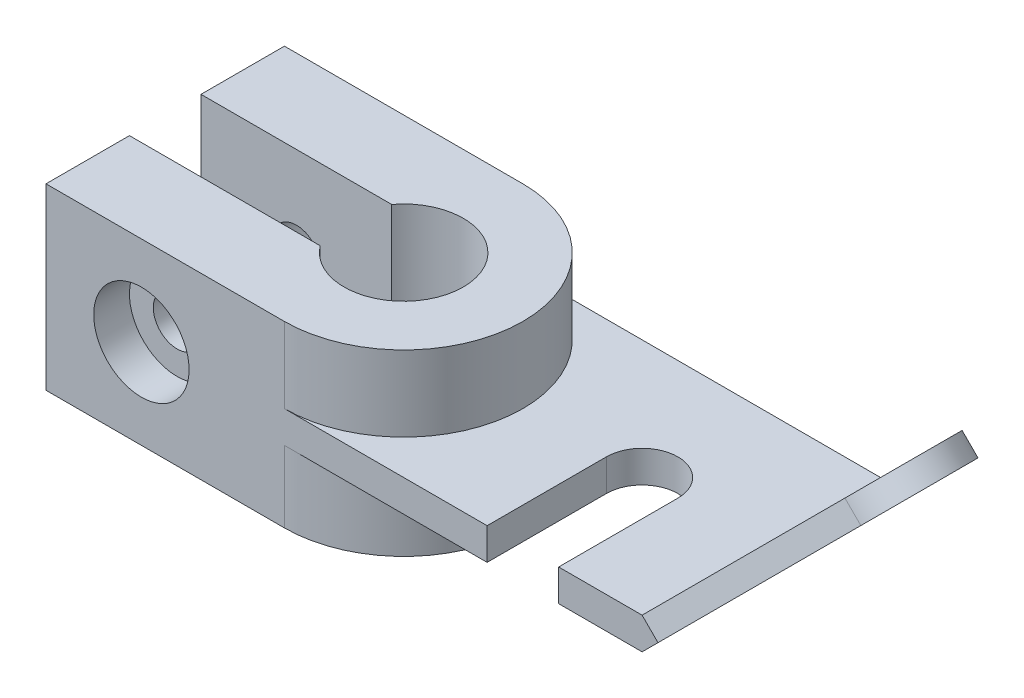
ISO-10303-21;
HEADER;
FILE_DESCRIPTION(('STEP AP214'),'2;1');
FILE_NAME('part.step','',(''),(''),'','','');
FILE_SCHEMA(('AUTOMOTIVE_DESIGN { 1 0 10303 214 1 1 1 1 }'));
ENDSEC;
DATA;
#1=APPLICATION_CONTEXT('core data for automotive mechanical design processes');
#2=APPLICATION_PROTOCOL_DEFINITION('international standard','automotive_design',2000,#1);
#3=PRODUCT_CONTEXT('',#1,'mechanical');
#4=PRODUCT('Part','Part','',(#3));
#5=PRODUCT_RELATED_PRODUCT_CATEGORY('part','',(#4));
#6=PRODUCT_DEFINITION_FORMATION('','',#4);
#7=PRODUCT_DEFINITION_CONTEXT('part definition',#1,'design');
#8=PRODUCT_DEFINITION('design','',#6,#7);
#9=PRODUCT_DEFINITION_SHAPE('','',#8);
#10=(LENGTH_UNIT() NAMED_UNIT(*) SI_UNIT(.MILLI.,.METRE.));
#11=(NAMED_UNIT(*) PLANE_ANGLE_UNIT() SI_UNIT($,.RADIAN.));
#12=(NAMED_UNIT(*) SI_UNIT($,.STERADIAN.) SOLID_ANGLE_UNIT());
#13=UNCERTAINTY_MEASURE_WITH_UNIT(LENGTH_MEASURE(1.E-05),#10,'distance_accuracy_value','');
#14=(GEOMETRIC_REPRESENTATION_CONTEXT(3) GLOBAL_UNCERTAINTY_ASSIGNED_CONTEXT((#13)) GLOBAL_UNIT_ASSIGNED_CONTEXT((#10,
#11,#12)) REPRESENTATION_CONTEXT('',''));
#15=CARTESIAN_POINT('',(0.,0.,0.));
#16=DIRECTION('',(0.,0.,1.));
#17=DIRECTION('',(1.,0.,0.));
#18=AXIS2_PLACEMENT_3D('',#15,#16,#17);
#19=CARTESIAN_POINT('',(0.,45.,-30.));
#20=DIRECTION('',(0.,0.,1.));
#21=DIRECTION('',(1.,0.,0.));
#22=AXIS2_PLACEMENT_3D('',#19,#20,#21);
#23=PLANE('',#22);
#24=DIRECTION('',(1.,0.,0.));
#25=VECTOR('',#24,1.);
#26=CARTESIAN_POINT('',(0.,26.,-30.));
#27=LINE('',#26,#25);
#28=CARTESIAN_POINT('',(0.,26.,-30.));
#29=VERTEX_POINT('',#28);
#30=CARTESIAN_POINT('',(90.,26.,-30.));
#31=VERTEX_POINT('',#30);
#32=EDGE_CURVE('E195',#29,#31,#27,.T.);
#33=ORIENTED_EDGE('',*,*,#32,.T.);
#34=DIRECTION('',(-0.707106781186544,0.707106781186551,0.));
#35=VECTOR('',#34,1.);
#36=CARTESIAN_POINT('',(96.3639610306789,19.636038969321,-30.));
#37=LINE('',#36,#35);
#38=CARTESIAN_POINT('',(94.,22.,-30.));
#39=VERTEX_POINT('',#38);
#40=EDGE_CURVE('E167',#39,#31,#37,.T.);
#41=ORIENTED_EDGE('',*,*,#40,.F.);
#42=DIRECTION('',(-0.707106781186551,-0.707106781186544,0.));
#43=VECTOR('',#42,1.);
#44=CARTESIAN_POINT('',(90.,18.,-30.));
#45=LINE('',#44,#43);
#46=CARTESIAN_POINT('',(90.,18.,-30.));
#47=VERTEX_POINT('',#46);
#48=EDGE_CURVE('E228',#39,#47,#45,.T.);
#49=ORIENTED_EDGE('',*,*,#48,.T.);
#50=DIRECTION('',(1.,0.,0.));
#51=VECTOR('',#50,1.);
#52=CARTESIAN_POINT('',(51.,18.,-30.));
#53=LINE('',#52,#51);
#54=CARTESIAN_POINT('',(0.,18.,-30.));
#55=VERTEX_POINT('',#54);
#56=EDGE_CURVE('E222',#55,#47,#53,.T.);
#57=ORIENTED_EDGE('',*,*,#56,.F.);
#58=DIRECTION('',(0.,-1.,0.));
#59=VECTOR('',#58,1.);
#60=CARTESIAN_POINT('',(0.,45.,-30.));
#61=LINE('',#60,#59);
#62=CARTESIAN_POINT('',(0.,0.,-30.));
#63=VERTEX_POINT('',#62);
#64=EDGE_CURVE('E303',#55,#63,#61,.T.);
#65=ORIENTED_EDGE('',*,*,#64,.T.);
#66=DIRECTION('',(-1.,0.,0.));
#67=VECTOR('',#66,1.);
#68=CARTESIAN_POINT('',(0.,0.,-30.));
#69=LINE('',#68,#67);
#70=CARTESIAN_POINT('',(-60.,0.,-30.));
#71=VERTEX_POINT('',#70);
#72=EDGE_CURVE('E279',#63,#71,#69,.T.);
#73=ORIENTED_EDGE('',*,*,#72,.T.);
#74=DIRECTION('',(0.,-1.,0.));
#75=VECTOR('',#74,1.);
#76=CARTESIAN_POINT('',(-60.,45.,-30.));
#77=LINE('',#76,#75);
#78=CARTESIAN_POINT('',(-60.,45.,-30.));
#79=VERTEX_POINT('',#78);
#80=EDGE_CURVE('E297',#79,#71,#77,.T.);
#81=ORIENTED_EDGE('',*,*,#80,.F.);
#82=DIRECTION('',(-1.,0.,0.));
#83=VECTOR('',#82,1.);
#84=CARTESIAN_POINT('',(0.,45.,-30.));
#85=LINE('',#84,#83);
#86=CARTESIAN_POINT('',(0.,45.,-30.));
#87=VERTEX_POINT('',#86);
#88=EDGE_CURVE('E260',#87,#79,#85,.T.);
#89=ORIENTED_EDGE('',*,*,#88,.F.);
#90=EDGE_CURVE('E197',#87,#29,#61,.T.);
#91=ORIENTED_EDGE('',*,*,#90,.T.);
#92=EDGE_LOOP('',(#33,#41,#49,#57,#65,#73,#81,#89,#91));
#93=FACE_BOUND('',#92,.T.);
#94=CARTESIAN_POINT('',(-36.,22.5,-30.));
#95=DIRECTION('',(0.,0.,-1.));
#96=DIRECTION('',(-1.,0.,0.));
#97=AXIS2_PLACEMENT_3D('',#94,#95,#96);
#98=CIRCLE('',#97,12.);
#99=CARTESIAN_POINT('',(-48.,22.5,-30.));
#100=VERTEX_POINT('',#99);
#101=EDGE_CURVE('E379',#100,#100,#98,.T.);
#102=ORIENTED_EDGE('',*,*,#101,.F.);
#103=EDGE_LOOP('',(#102));
#104=FACE_BOUND('',#103,.T.);
#105=ADVANCED_FACE('F41',(#93,#104),#23,.F.);
#106=CARTESIAN_POINT('',(0.,45.,0.));
#107=DIRECTION('',(0.,-1.,0.));
#108=DIRECTION('',(0.,0.,-1.));
#109=AXIS2_PLACEMENT_3D('',#106,#107,#108);
#110=CYLINDRICAL_SURFACE('',#109,30.);
#111=CARTESIAN_POINT('',(0.,26.,0.));
#112=DIRECTION('',(0.,1.,0.));
#113=DIRECTION('',(0.,0.,-1.));
#114=AXIS2_PLACEMENT_3D('',#111,#112,#113);
#115=CIRCLE('',#114,30.);
#116=CARTESIAN_POINT('',(0.,26.,30.));
#117=VERTEX_POINT('',#116);
#118=EDGE_CURVE('E200',#117,#29,#115,.T.);
#119=ORIENTED_EDGE('',*,*,#118,.T.);
#120=ORIENTED_EDGE('',*,*,#90,.F.);
#121=CARTESIAN_POINT('',(0.,45.,0.));
#122=DIRECTION('',(0.,1.,0.));
#123=DIRECTION('',(0.,0.,1.));
#124=AXIS2_PLACEMENT_3D('',#121,#122,#123);
#125=CIRCLE('',#124,30.);
#126=CARTESIAN_POINT('',(0.,45.,30.));
#127=VERTEX_POINT('',#126);
#128=EDGE_CURVE('E253',#127,#87,#125,.T.);
#129=ORIENTED_EDGE('',*,*,#128,.F.);
#130=DIRECTION('',(0.,-1.,0.));
#131=VECTOR('',#130,1.);
#132=CARTESIAN_POINT('',(0.,45.,30.));
#133=LINE('',#132,#131);
#134=EDGE_CURVE('E306',#127,#117,#133,.T.);
#135=ORIENTED_EDGE('',*,*,#134,.T.);
#136=EDGE_LOOP('',(#119,#120,#129,#135));
#137=FACE_BOUND('',#136,.T.);
#138=ADVANCED_FACE('F322',(#137),#110,.T.);
#139=CARTESIAN_POINT('',(0.,45.,30.));
#140=DIRECTION('',(0.,0.,1.));
#141=DIRECTION('',(1.,0.,0.));
#142=AXIS2_PLACEMENT_3D('',#139,#140,#141);
#143=PLANE('',#142);
#144=CARTESIAN_POINT('',(-36.,22.5,30.));
#145=DIRECTION('',(0.,0.,1.));
#146=DIRECTION('',(1.,0.,0.));
#147=AXIS2_PLACEMENT_3D('',#144,#145,#146);
#148=CIRCLE('',#147,12.);
#149=CARTESIAN_POINT('',(-24.,22.5,30.));
#150=VERTEX_POINT('',#149);
#151=EDGE_CURVE('E368',#150,#150,#148,.T.);
#152=ORIENTED_EDGE('',*,*,#151,.F.);
#153=EDGE_LOOP('',(#152));
#154=FACE_BOUND('',#153,.T.);
#155=DIRECTION('',(-1.,0.,0.));
#156=VECTOR('',#155,1.);
#157=CARTESIAN_POINT('',(0.,0.,30.));
#158=LINE('',#157,#156);
#159=CARTESIAN_POINT('',(0.,0.,30.));
#160=VERTEX_POINT('',#159);
#161=CARTESIAN_POINT('',(-60.,0.,30.));
#162=VERTEX_POINT('',#161);
#163=EDGE_CURVE('E246',#160,#162,#158,.T.);
#164=ORIENTED_EDGE('',*,*,#163,.F.);
#165=CARTESIAN_POINT('',(0.,18.,30.));
#166=VERTEX_POINT('',#165);
#167=EDGE_CURVE('E304',#166,#160,#133,.T.);
#168=ORIENTED_EDGE('',*,*,#167,.F.);
#169=DIRECTION('',(-1.,0.,0.));
#170=VECTOR('',#169,1.);
#171=CARTESIAN_POINT('',(0.,18.,30.));
#172=LINE('',#171,#170);
#173=CARTESIAN_POINT('',(51.,18.,30.));
#174=VERTEX_POINT('',#173);
#175=EDGE_CURVE('E245',#174,#166,#172,.T.);
#176=ORIENTED_EDGE('',*,*,#175,.F.);
#177=DIRECTION('',(0.,-1.,0.));
#178=VECTOR('',#177,1.);
#179=CARTESIAN_POINT('',(51.,26.,30.));
#180=LINE('',#179,#178);
#181=CARTESIAN_POINT('',(51.,26.,30.));
#182=VERTEX_POINT('',#181);
#183=EDGE_CURVE('E242',#182,#174,#180,.T.);
#184=ORIENTED_EDGE('',*,*,#183,.F.);
#185=DIRECTION('',(-1.,0.,0.));
#186=VECTOR('',#185,1.);
#187=CARTESIAN_POINT('',(0.,26.,30.));
#188=LINE('',#187,#186);
#189=EDGE_CURVE('E220',#182,#117,#188,.T.);
#190=ORIENTED_EDGE('',*,*,#189,.T.);
#191=ORIENTED_EDGE('',*,*,#134,.F.);
#192=DIRECTION('',(-1.,0.,0.));
#193=VECTOR('',#192,1.);
#194=CARTESIAN_POINT('',(0.,45.,30.));
#195=LINE('',#194,#193);
#196=CARTESIAN_POINT('',(-60.,45.,30.));
#197=VERTEX_POINT('',#196);
#198=EDGE_CURVE('E255',#127,#197,#195,.T.);
#199=ORIENTED_EDGE('',*,*,#198,.T.);
#200=DIRECTION('',(0.,-1.,0.));
#201=VECTOR('',#200,1.);
#202=CARTESIAN_POINT('',(-60.,45.,30.));
#203=LINE('',#202,#201);
#204=EDGE_CURVE('E289',#197,#162,#203,.T.);
#205=ORIENTED_EDGE('',*,*,#204,.T.);
#206=EDGE_LOOP('',(#164,#168,#176,#184,#190,#191,#199,#205));
#207=FACE_BOUND('',#206,.T.);
#208=ADVANCED_FACE('F43',(#154,#207),#143,.T.);
#209=ORIENTED_EDGE('',*,*,#64,.F.);
#210=CARTESIAN_POINT('',(0.,18.,0.));
#211=DIRECTION('',(0.,1.,0.));
#212=DIRECTION('',(0.,0.,-1.));
#213=AXIS2_PLACEMENT_3D('',#210,#211,#212);
#214=CIRCLE('',#213,30.);
#215=EDGE_CURVE('E63',#166,#55,#214,.T.);
#216=ORIENTED_EDGE('',*,*,#215,.F.);
#217=ORIENTED_EDGE('',*,*,#167,.T.);
#218=CARTESIAN_POINT('',(0.,0.,0.));
#219=DIRECTION('',(0.,1.,0.));
#220=DIRECTION('',(0.,0.,1.));
#221=AXIS2_PLACEMENT_3D('',#218,#219,#220);
#222=CIRCLE('',#221,30.);
#223=EDGE_CURVE('E271',#160,#63,#222,.T.);
#224=ORIENTED_EDGE('',*,*,#223,.T.);
#225=EDGE_LOOP('',(#209,#216,#217,#224));
#226=FACE_BOUND('',#225,.T.);
#227=ADVANCED_FACE('F392',(#226),#110,.T.);
#228=CARTESIAN_POINT('',(-60.,45.,0.));
#229=DIRECTION('',(1.,0.,0.));
#230=DIRECTION('',(0.,0.,-1.));
#231=AXIS2_PLACEMENT_3D('',#228,#229,#230);
#232=PLANE('',#231);
#233=DIRECTION('',(0.,0.,1.));
#234=VECTOR('',#233,1.);
#235=CARTESIAN_POINT('',(-60.,0.,0.));
#236=LINE('',#235,#234);
#237=CARTESIAN_POINT('',(-60.,0.,-9.));
#238=VERTEX_POINT('',#237);
#239=EDGE_CURVE('E280',#71,#238,#236,.T.);
#240=ORIENTED_EDGE('',*,*,#239,.T.);
#241=DIRECTION('',(0.,-1.,0.));
#242=VECTOR('',#241,1.);
#243=CARTESIAN_POINT('',(-60.,45.,-9.));
#244=LINE('',#243,#242);
#245=CARTESIAN_POINT('',(-60.,45.,-9.));
#246=VERTEX_POINT('',#245);
#247=EDGE_CURVE('E300',#246,#238,#244,.T.);
#248=ORIENTED_EDGE('',*,*,#247,.F.);
#249=DIRECTION('',(0.,0.,1.));
#250=VECTOR('',#249,1.);
#251=CARTESIAN_POINT('',(-60.,45.,0.));
#252=LINE('',#251,#250);
#253=EDGE_CURVE('E257',#79,#246,#252,.T.);
#254=ORIENTED_EDGE('',*,*,#253,.F.);
#255=ORIENTED_EDGE('',*,*,#80,.T.);
#256=EDGE_LOOP('',(#240,#248,#254,#255));
#257=FACE_BOUND('',#256,.T.);
#258=ADVANCED_FACE('F400',(#257),#232,.F.);
#259=CARTESIAN_POINT('',(0.,45.,-9.));
#260=DIRECTION('',(0.,0.,-1.));
#261=DIRECTION('',(-1.,0.,0.));
#262=AXIS2_PLACEMENT_3D('',#259,#260,#261);
#263=PLANE('',#262);
#264=CARTESIAN_POINT('',(-36.,22.5,-9.));
#265=DIRECTION('',(0.,0.,-1.));
#266=DIRECTION('',(-1.,0.,0.));
#267=AXIS2_PLACEMENT_3D('',#264,#265,#266);
#268=CIRCLE('',#267,6.);
#269=CARTESIAN_POINT('',(-42.,22.5,-9.));
#270=VERTEX_POINT('',#269);
#271=EDGE_CURVE('E371',#270,#270,#268,.T.);
#272=ORIENTED_EDGE('',*,*,#271,.T.);
#273=EDGE_LOOP('',(#272));
#274=FACE_BOUND('',#273,.T.);
#275=DIRECTION('',(1.,0.,0.));
#276=VECTOR('',#275,1.);
#277=CARTESIAN_POINT('',(0.,0.,-9.));
#278=LINE('',#277,#276);
#279=CARTESIAN_POINT('',(-12.,0.,-9.));
#280=VERTEX_POINT('',#279);
#281=EDGE_CURVE('E277',#238,#280,#278,.T.);
#282=ORIENTED_EDGE('',*,*,#281,.T.);
#283=DIRECTION('',(0.,-1.,0.));
#284=VECTOR('',#283,1.);
#285=CARTESIAN_POINT('',(-12.,45.,-9.));
#286=LINE('',#285,#284);
#287=CARTESIAN_POINT('',(-12.,45.,-9.));
#288=VERTEX_POINT('',#287);
#289=EDGE_CURVE('E294',#288,#280,#286,.T.);
#290=ORIENTED_EDGE('',*,*,#289,.F.);
#291=DIRECTION('',(1.,0.,0.));
#292=VECTOR('',#291,1.);
#293=CARTESIAN_POINT('',(0.,45.,-9.));
#294=LINE('',#293,#292);
#295=EDGE_CURVE('E262',#246,#288,#294,.T.);
#296=ORIENTED_EDGE('',*,*,#295,.F.);
#297=ORIENTED_EDGE('',*,*,#247,.T.);
#298=EDGE_LOOP('',(#282,#290,#296,#297));
#299=FACE_BOUND('',#298,.T.);
#300=ADVANCED_FACE('F393',(#274,#299),#263,.F.);
#301=CARTESIAN_POINT('',(0.,45.,0.));
#302=DIRECTION('',(0.,-1.,0.));
#303=DIRECTION('',(0.,0.,-1.));
#304=AXIS2_PLACEMENT_3D('',#301,#302,#303);
#305=CYLINDRICAL_SURFACE('',#304,15.);
#306=CARTESIAN_POINT('',(0.,0.,0.));
#307=DIRECTION('',(0.,1.,0.));
#308=DIRECTION('',(0.,0.,1.));
#309=AXIS2_PLACEMENT_3D('',#306,#307,#308);
#310=CIRCLE('',#309,15.);
#311=CARTESIAN_POINT('',(-12.,0.,9.));
#312=VERTEX_POINT('',#311);
#313=EDGE_CURVE('E284',#312,#280,#310,.T.);
#314=ORIENTED_EDGE('',*,*,#313,.F.);
#315=DIRECTION('',(0.,-1.,0.));
#316=VECTOR('',#315,1.);
#317=CARTESIAN_POINT('',(-12.,45.,9.));
#318=LINE('',#317,#316);
#319=CARTESIAN_POINT('',(-12.,45.,9.));
#320=VERTEX_POINT('',#319);
#321=EDGE_CURVE('E291',#320,#312,#318,.T.);
#322=ORIENTED_EDGE('',*,*,#321,.F.);
#323=CARTESIAN_POINT('',(0.,45.,0.));
#324=DIRECTION('',(0.,1.,0.));
#325=DIRECTION('',(0.,0.,1.));
#326=AXIS2_PLACEMENT_3D('',#323,#324,#325);
#327=CIRCLE('',#326,15.);
#328=EDGE_CURVE('E265',#320,#288,#327,.T.);
#329=ORIENTED_EDGE('',*,*,#328,.T.);
#330=ORIENTED_EDGE('',*,*,#289,.T.);
#331=EDGE_LOOP('',(#314,#322,#329,#330));
#332=FACE_BOUND('',#331,.T.);
#333=ADVANCED_FACE('F452',(#332),#305,.F.);
#334=CARTESIAN_POINT('',(0.,45.,9.));
#335=DIRECTION('',(0.,0.,-1.));
#336=DIRECTION('',(-1.,0.,0.));
#337=AXIS2_PLACEMENT_3D('',#334,#335,#336);
#338=PLANE('',#337);
#339=CARTESIAN_POINT('',(-36.,22.5,9.));
#340=DIRECTION('',(0.,0.,-1.));
#341=DIRECTION('',(-1.,0.,0.));
#342=AXIS2_PLACEMENT_3D('',#339,#340,#341);
#343=CIRCLE('',#342,6.);
#344=CARTESIAN_POINT('',(-42.,22.5,9.));
#345=VERTEX_POINT('',#344);
#346=EDGE_CURVE('E360',#345,#345,#343,.T.);
#347=ORIENTED_EDGE('',*,*,#346,.F.);
#348=EDGE_LOOP('',(#347));
#349=FACE_BOUND('',#348,.T.);
#350=DIRECTION('',(1.,0.,0.));
#351=VECTOR('',#350,1.);
#352=CARTESIAN_POINT('',(0.,0.,9.));
#353=LINE('',#352,#351);
#354=CARTESIAN_POINT('',(-60.,0.,9.00000000000001));
#355=VERTEX_POINT('',#354);
#356=EDGE_CURVE('E288',#355,#312,#353,.T.);
#357=ORIENTED_EDGE('',*,*,#356,.F.);
#358=DIRECTION('',(0.,-1.,0.));
#359=VECTOR('',#358,1.);
#360=CARTESIAN_POINT('',(-60.,45.,9.00000000000001));
#361=LINE('',#360,#359);
#362=CARTESIAN_POINT('',(-60.,45.,9.00000000000001));
#363=VERTEX_POINT('',#362);
#364=EDGE_CURVE('E293',#363,#355,#361,.T.);
#365=ORIENTED_EDGE('',*,*,#364,.F.);
#366=DIRECTION('',(1.,0.,0.));
#367=VECTOR('',#366,1.);
#368=CARTESIAN_POINT('',(0.,45.,9.));
#369=LINE('',#368,#367);
#370=EDGE_CURVE('E266',#363,#320,#369,.T.);
#371=ORIENTED_EDGE('',*,*,#370,.T.);
#372=ORIENTED_EDGE('',*,*,#321,.T.);
#373=EDGE_LOOP('',(#357,#365,#371,#372));
#374=FACE_BOUND('',#373,.T.);
#375=ADVANCED_FACE('F451',(#349,#374),#338,.T.);
#376=EDGE_CURVE('E259',#355,#162,#236,.T.);
#377=ORIENTED_EDGE('',*,*,#376,.T.);
#378=ORIENTED_EDGE('',*,*,#204,.F.);
#379=EDGE_CURVE('E264',#363,#197,#252,.T.);
#380=ORIENTED_EDGE('',*,*,#379,.F.);
#381=ORIENTED_EDGE('',*,*,#364,.T.);
#382=EDGE_LOOP('',(#377,#378,#380,#381));
#383=FACE_BOUND('',#382,.T.);
#384=ADVANCED_FACE('F403',(#383),#232,.F.);
#385=CARTESIAN_POINT('',(0.,45.,0.));
#386=DIRECTION('',(0.,1.,0.));
#387=DIRECTION('',(0.,0.,1.));
#388=AXIS2_PLACEMENT_3D('',#385,#386,#387);
#389=PLANE('',#388);
#390=ORIENTED_EDGE('',*,*,#198,.F.);
#391=ORIENTED_EDGE('',*,*,#128,.T.);
#392=ORIENTED_EDGE('',*,*,#88,.T.);
#393=ORIENTED_EDGE('',*,*,#253,.T.);
#394=ORIENTED_EDGE('',*,*,#295,.T.);
#395=ORIENTED_EDGE('',*,*,#328,.F.);
#396=ORIENTED_EDGE('',*,*,#370,.F.);
#397=ORIENTED_EDGE('',*,*,#379,.T.);
#398=EDGE_LOOP('',(#390,#391,#392,#393,#394,#395,#396,#397));
#399=FACE_BOUND('',#398,.T.);
#400=ADVANCED_FACE('F443',(#399),#389,.T.);
#401=CARTESIAN_POINT('',(0.,0.,0.));
#402=DIRECTION('',(0.,1.,0.));
#403=DIRECTION('',(0.,0.,1.));
#404=AXIS2_PLACEMENT_3D('',#401,#402,#403);
#405=PLANE('',#404);
#406=ORIENTED_EDGE('',*,*,#163,.T.);
#407=ORIENTED_EDGE('',*,*,#376,.F.);
#408=ORIENTED_EDGE('',*,*,#356,.T.);
#409=ORIENTED_EDGE('',*,*,#313,.T.);
#410=ORIENTED_EDGE('',*,*,#281,.F.);
#411=ORIENTED_EDGE('',*,*,#239,.F.);
#412=ORIENTED_EDGE('',*,*,#72,.F.);
#413=ORIENTED_EDGE('',*,*,#223,.F.);
#414=EDGE_LOOP('',(#406,#407,#408,#409,#410,#411,#412,#413));
#415=FACE_BOUND('',#414,.T.);
#416=ADVANCED_FACE('F440',(#415),#405,.F.);
#417=CARTESIAN_POINT('',(51.,26.,0.));
#418=DIRECTION('',(1.,0.,0.));
#419=DIRECTION('',(0.,0.,-1.));
#420=AXIS2_PLACEMENT_3D('',#417,#418,#419);
#421=PLANE('',#420);
#422=DIRECTION('',(0.,0.,1.));
#423=VECTOR('',#422,1.);
#424=CARTESIAN_POINT('',(51.,18.,0.));
#425=LINE('',#424,#423);
#426=CARTESIAN_POINT('',(51.,18.,0.));
#427=VERTEX_POINT('',#426);
#428=EDGE_CURVE('E237',#427,#174,#425,.T.);
#429=ORIENTED_EDGE('',*,*,#428,.F.);
#430=DIRECTION('',(0.,-1.,0.));
#431=VECTOR('',#430,1.);
#432=CARTESIAN_POINT('',(51.,26.,0.));
#433=LINE('',#432,#431);
#434=CARTESIAN_POINT('',(51.,26.,0.));
#435=VERTEX_POINT('',#434);
#436=EDGE_CURVE('E250',#435,#427,#433,.T.);
#437=ORIENTED_EDGE('',*,*,#436,.F.);
#438=DIRECTION('',(0.,0.,1.));
#439=VECTOR('',#438,1.);
#440=CARTESIAN_POINT('',(51.,26.,0.));
#441=LINE('',#440,#439);
#442=EDGE_CURVE('E217',#435,#182,#441,.T.);
#443=ORIENTED_EDGE('',*,*,#442,.T.);
#444=ORIENTED_EDGE('',*,*,#183,.T.);
#445=EDGE_LOOP('',(#429,#437,#443,#444));
#446=FACE_BOUND('',#445,.T.);
#447=ADVANCED_FACE('F332',(#446),#421,.T.);
#448=CARTESIAN_POINT('',(60.,26.,0.));
#449=DIRECTION('',(0.,-1.,0.));
#450=DIRECTION('',(0.,0.,-1.));
#451=AXIS2_PLACEMENT_3D('',#448,#449,#450);
#452=CYLINDRICAL_SURFACE('',#451,9.00000000000001);
#453=CARTESIAN_POINT('',(60.,18.,0.));
#454=DIRECTION('',(0.,1.,0.));
#455=DIRECTION('',(0.,0.,-1.));
#456=AXIS2_PLACEMENT_3D('',#453,#454,#455);
#457=CIRCLE('',#456,9.00000000000001);
#458=CARTESIAN_POINT('',(69.,18.,0.));
#459=VERTEX_POINT('',#458);
#460=EDGE_CURVE('E236',#459,#427,#457,.T.);
#461=ORIENTED_EDGE('',*,*,#460,.F.);
#462=DIRECTION('',(0.,-1.,0.));
#463=VECTOR('',#462,1.);
#464=CARTESIAN_POINT('',(69.,26.,0.));
#465=LINE('',#464,#463);
#466=CARTESIAN_POINT('',(69.,26.,0.));
#467=VERTEX_POINT('',#466);
#468=EDGE_CURVE('E248',#467,#459,#465,.T.);
#469=ORIENTED_EDGE('',*,*,#468,.F.);
#470=CARTESIAN_POINT('',(60.,26.,0.));
#471=DIRECTION('',(0.,1.,0.));
#472=DIRECTION('',(0.,0.,-1.));
#473=AXIS2_PLACEMENT_3D('',#470,#471,#472);
#474=CIRCLE('',#473,9.00000000000001);
#475=EDGE_CURVE('E213',#467,#435,#474,.T.);
#476=ORIENTED_EDGE('',*,*,#475,.T.);
#477=ORIENTED_EDGE('',*,*,#436,.T.);
#478=EDGE_LOOP('',(#461,#469,#476,#477));
#479=FACE_BOUND('',#478,.T.);
#480=ADVANCED_FACE('F339',(#479),#452,.F.);
#481=CARTESIAN_POINT('',(69.,26.,0.));
#482=DIRECTION('',(-1.,0.,0.));
#483=DIRECTION('',(0.,0.,1.));
#484=AXIS2_PLACEMENT_3D('',#481,#482,#483);
#485=PLANE('',#484);
#486=DIRECTION('',(0.,0.,-1.));
#487=VECTOR('',#486,1.);
#488=CARTESIAN_POINT('',(69.,18.,0.));
#489=LINE('',#488,#487);
#490=CARTESIAN_POINT('',(69.,18.,30.));
#491=VERTEX_POINT('',#490);
#492=EDGE_CURVE('E231',#491,#459,#489,.T.);
#493=ORIENTED_EDGE('',*,*,#492,.F.);
#494=DIRECTION('',(0.,-1.,0.));
#495=VECTOR('',#494,1.);
#496=CARTESIAN_POINT('',(69.,26.,30.));
#497=LINE('',#496,#495);
#498=CARTESIAN_POINT('',(69.,26.,30.));
#499=VERTEX_POINT('',#498);
#500=EDGE_CURVE('E221',#499,#491,#497,.T.);
#501=ORIENTED_EDGE('',*,*,#500,.F.);
#502=DIRECTION('',(0.,0.,-1.));
#503=VECTOR('',#502,1.);
#504=CARTESIAN_POINT('',(69.,26.,0.));
#505=LINE('',#504,#503);
#506=EDGE_CURVE('E206',#499,#467,#505,.T.);
#507=ORIENTED_EDGE('',*,*,#506,.T.);
#508=ORIENTED_EDGE('',*,*,#468,.T.);
#509=EDGE_LOOP('',(#493,#501,#507,#508));
#510=FACE_BOUND('',#509,.T.);
#511=ADVANCED_FACE('F341',(#510),#485,.T.);
#512=CARTESIAN_POINT('',(69.,26.,30.));
#513=DIRECTION('',(0.,0.,1.));
#514=DIRECTION('',(1.,0.,0.));
#515=AXIS2_PLACEMENT_3D('',#512,#513,#514);
#516=PLANE('',#515);
#517=DIRECTION('',(-0.707106781186544,0.707106781186551,0.));
#518=VECTOR('',#517,1.);
#519=CARTESIAN_POINT('',(96.3639610306789,19.636038969321,30.));
#520=LINE('',#519,#518);
#521=CARTESIAN_POINT('',(94.,22.,30.));
#522=VERTEX_POINT('',#521);
#523=CARTESIAN_POINT('',(90.,26.,30.));
#524=VERTEX_POINT('',#523);
#525=EDGE_CURVE('E321',#522,#524,#520,.T.);
#526=ORIENTED_EDGE('',*,*,#525,.T.);
#527=DIRECTION('',(-1.,0.,0.));
#528=VECTOR('',#527,1.);
#529=CARTESIAN_POINT('',(69.,26.,30.));
#530=LINE('',#529,#528);
#531=EDGE_CURVE('E207',#524,#499,#530,.T.);
#532=ORIENTED_EDGE('',*,*,#531,.T.);
#533=ORIENTED_EDGE('',*,*,#500,.T.);
#534=DIRECTION('',(-1.,0.,0.));
#535=VECTOR('',#534,1.);
#536=CARTESIAN_POINT('',(69.,18.,30.));
#537=LINE('',#536,#535);
#538=CARTESIAN_POINT('',(90.,18.,30.));
#539=VERTEX_POINT('',#538);
#540=EDGE_CURVE('E229',#539,#491,#537,.T.);
#541=ORIENTED_EDGE('',*,*,#540,.F.);
#542=DIRECTION('',(0.707106781186551,0.707106781186544,0.));
#543=VECTOR('',#542,1.);
#544=CARTESIAN_POINT('',(90.,18.,30.));
#545=LINE('',#544,#543);
#546=EDGE_CURVE('E316',#539,#522,#545,.T.);
#547=ORIENTED_EDGE('',*,*,#546,.T.);
#548=EDGE_LOOP('',(#526,#532,#533,#541,#547));
#549=FACE_BOUND('',#548,.T.);
#550=ADVANCED_FACE('F342',(#549),#516,.T.);
#551=CARTESIAN_POINT('',(0.,26.,0.));
#552=DIRECTION('',(0.,-1.,0.));
#553=DIRECTION('',(0.,0.,-1.));
#554=AXIS2_PLACEMENT_3D('',#551,#552,#553);
#555=PLANE('',#554);
#556=ORIENTED_EDGE('',*,*,#118,.F.);
#557=ORIENTED_EDGE('',*,*,#189,.F.);
#558=ORIENTED_EDGE('',*,*,#442,.F.);
#559=ORIENTED_EDGE('',*,*,#475,.F.);
#560=ORIENTED_EDGE('',*,*,#506,.F.);
#561=ORIENTED_EDGE('',*,*,#531,.F.);
#562=DIRECTION('',(0.,0.,1.));
#563=VECTOR('',#562,1.);
#564=CARTESIAN_POINT('',(90.,26.,-30.));
#565=LINE('',#564,#563);
#566=EDGE_CURVE('E190',#31,#524,#565,.T.);
#567=ORIENTED_EDGE('',*,*,#566,.F.);
#568=ORIENTED_EDGE('',*,*,#32,.F.);
#569=EDGE_LOOP('',(#556,#557,#558,#559,#560,#561,#567,#568));
#570=FACE_BOUND('',#569,.T.);
#571=ADVANCED_FACE('F201',(#570),#555,.F.);
#572=CARTESIAN_POINT('',(0.,18.,0.));
#573=DIRECTION('',(0.,-1.,0.));
#574=DIRECTION('',(0.,0.,-1.));
#575=AXIS2_PLACEMENT_3D('',#572,#573,#574);
#576=PLANE('',#575);
#577=ORIENTED_EDGE('',*,*,#215,.T.);
#578=ORIENTED_EDGE('',*,*,#56,.T.);
#579=DIRECTION('',(0.,0.,1.));
#580=VECTOR('',#579,1.);
#581=CARTESIAN_POINT('',(90.,18.,-30.));
#582=LINE('',#581,#580);
#583=EDGE_CURVE('E226',#47,#539,#582,.T.);
#584=ORIENTED_EDGE('',*,*,#583,.T.);
#585=ORIENTED_EDGE('',*,*,#540,.T.);
#586=ORIENTED_EDGE('',*,*,#492,.T.);
#587=ORIENTED_EDGE('',*,*,#460,.T.);
#588=ORIENTED_EDGE('',*,*,#428,.T.);
#589=ORIENTED_EDGE('',*,*,#175,.T.);
#590=EDGE_LOOP('',(#577,#578,#584,#585,#586,#587,#588,#589));
#591=FACE_BOUND('',#590,.T.);
#592=ADVANCED_FACE('F412',(#591),#576,.T.);
#593=CARTESIAN_POINT('',(90.,26.,-99.3541635375985));
#594=DIRECTION('',(-0.707106781186544,0.707106781186551,0.));
#595=DIRECTION('',(-0.707106781186551,-0.707106781186544,0.));
#596=AXIS2_PLACEMENT_3D('',#593,#594,#595);
#597=PLANE('',#596);
#598=CARTESIAN_POINT('',(122.173358543988,58.1733585439878,0.));
#599=DIRECTION('',(-0.707106781186544,0.707106781186551,0.));
#600=DIRECTION('',(-0.707106781186551,-0.707106781186544,0.));
#601=AXIS2_PLACEMENT_3D('',#598,#599,#600);
#602=CIRCLE('',#601,7.49999999999999);
#603=CARTESIAN_POINT('',(116.870057685089,52.8700576850887,0.));
#604=VERTEX_POINT('',#603);
#605=EDGE_CURVE('E358',#604,#604,#602,.T.);
#606=ORIENTED_EDGE('',*,*,#605,.F.);
#607=EDGE_LOOP('',(#606));
#608=FACE_BOUND('',#607,.T.);
#609=DIRECTION('',(-0.674665588129943,-0.674665588129936,0.299420587780075));
#610=VECTOR('',#609,1.);
#611=CARTESIAN_POINT('',(125.34919346468,61.34919346468,14.3118183719967));
#612=LINE('',#611,#610);
#613=CARTESIAN_POINT('',(125.34919346468,61.34919346468,14.3118183719967));
#614=VERTEX_POINT('',#613);
#615=EDGE_CURVE('E179',#614,#524,#612,.T.);
#616=ORIENTED_EDGE('',*,*,#615,.F.);
#617=CARTESIAN_POINT('',(122.173358543988,58.1733585439878,0.));
#618=DIRECTION('',(0.707106781186544,-0.707106781186551,0.));
#619=DIRECTION('',(-0.707106781186551,-0.707106781186544,0.));
#620=AXIS2_PLACEMENT_3D('',#617,#618,#619);
#621=CIRCLE('',#620,15.);
#622=CARTESIAN_POINT('',(125.34919346468,61.34919346468,-14.3118183719967));
#623=VERTEX_POINT('',#622);
#624=EDGE_CURVE('E186',#623,#614,#621,.T.);
#625=ORIENTED_EDGE('',*,*,#624,.F.);
#626=DIRECTION('',(0.674665588129943,0.674665588129936,0.299420587780075));
#627=VECTOR('',#626,1.);
#628=CARTESIAN_POINT('',(125.34919346468,61.34919346468,-14.3118183719967));
#629=LINE('',#628,#627);
#630=EDGE_CURVE('E173',#31,#623,#629,.T.);
#631=ORIENTED_EDGE('',*,*,#630,.F.);
#632=ORIENTED_EDGE('',*,*,#566,.T.);
#633=EDGE_LOOP('',(#616,#625,#631,#632));
#634=FACE_BOUND('',#633,.T.);
#635=ADVANCED_FACE('F184',(#608,#634),#597,.T.);
#636=CARTESIAN_POINT('',(90.,18.,-99.3541635375985));
#637=DIRECTION('',(0.707106781186544,-0.707106781186551,0.));
#638=DIRECTION('',(0.707106781186551,0.707106781186544,0.));
#639=AXIS2_PLACEMENT_3D('',#636,#637,#638);
#640=PLANE('',#639);
#641=CARTESIAN_POINT('',(126.173358543988,54.1733585439877,0.));
#642=DIRECTION('',(0.707106781186544,-0.707106781186551,0.));
#643=DIRECTION('',(0.707106781186551,0.707106781186544,0.));
#644=AXIS2_PLACEMENT_3D('',#641,#642,#643);
#645=CIRCLE('',#644,7.49999999999999);
#646=CARTESIAN_POINT('',(131.476659402887,59.4766594028868,0.));
#647=VERTEX_POINT('',#646);
#648=EDGE_CURVE('E188',#647,#647,#645,.T.);
#649=ORIENTED_EDGE('',*,*,#648,.F.);
#650=EDGE_LOOP('',(#649));
#651=FACE_BOUND('',#650,.T.);
#652=DIRECTION('',(0.674665588129943,0.674665588129936,-0.299420587780075));
#653=VECTOR('',#652,1.);
#654=CARTESIAN_POINT('',(116.489285829995,44.4892858299946,20.0191216204817));
#655=LINE('',#654,#653);
#656=CARTESIAN_POINT('',(129.34919346468,57.34919346468,14.3118183719967));
#657=VERTEX_POINT('',#656);
#658=EDGE_CURVE('E11',#522,#657,#655,.T.);
#659=ORIENTED_EDGE('',*,*,#658,.F.);
#660=ORIENTED_EDGE('',*,*,#546,.F.);
#661=ORIENTED_EDGE('',*,*,#583,.F.);
#662=ORIENTED_EDGE('',*,*,#48,.F.);
#663=DIRECTION('',(-0.674665588129943,-0.674665588129936,-0.299420587780075));
#664=VECTOR('',#663,1.);
#665=CARTESIAN_POINT('',(76.3484616942691,4.3484616942693,-37.8338573475701));
#666=LINE('',#665,#664);
#667=CARTESIAN_POINT('',(129.34919346468,57.34919346468,-14.3118183719967));
#668=VERTEX_POINT('',#667);
#669=EDGE_CURVE('E176',#668,#39,#666,.T.);
#670=ORIENTED_EDGE('',*,*,#669,.F.);
#671=CARTESIAN_POINT('',(126.173358543988,54.1733585439877,0.));
#672=DIRECTION('',(0.707106781186544,-0.707106781186551,0.));
#673=DIRECTION('',(0.707106781186551,0.707106781186544,0.));
#674=AXIS2_PLACEMENT_3D('',#671,#672,#673);
#675=CIRCLE('',#674,15.);
#676=EDGE_CURVE('E47',#657,#668,#675,.F.);
#677=ORIENTED_EDGE('',*,*,#676,.F.);
#678=EDGE_LOOP('',(#659,#660,#661,#662,#670,#677));
#679=FACE_BOUND('',#678,.T.);
#680=ADVANCED_FACE('F317',(#651,#679),#640,.T.);
#681=CARTESIAN_POINT('',(131.713154495359,54.9852324340011,14.3118183719967));
#682=DIRECTION('',(-0.211722328046154,-0.211722328046152,-0.954121224799781));
#683=DIRECTION('',(-0.976253017093471,0.,0.216633438360504));
#684=AXIS2_PLACEMENT_3D('',#681,#682,#683);
#685=PLANE('',#684);
#686=ORIENTED_EDGE('',*,*,#658,.T.);
#687=DIRECTION('',(-0.707106781186544,0.707106781186551,0.));
#688=VECTOR('',#687,1.);
#689=CARTESIAN_POINT('',(131.713154495359,54.9852324340011,14.3118183719967));
#690=LINE('',#689,#688);
#691=EDGE_CURVE('E312',#657,#614,#690,.T.);
#692=ORIENTED_EDGE('',*,*,#691,.T.);
#693=ORIENTED_EDGE('',*,*,#615,.T.);
#694=ORIENTED_EDGE('',*,*,#525,.F.);
#695=EDGE_LOOP('',(#686,#692,#693,#694));
#696=FACE_BOUND('',#695,.T.);
#697=ADVANCED_FACE('F414',(#696),#685,.F.);
#698=CARTESIAN_POINT('',(128.537319574667,51.8093975133088,0.));
#699=DIRECTION('',(-0.707106781186544,0.707106781186551,0.));
#700=DIRECTION('',(-0.707106781186551,-0.707106781186544,0.));
#701=AXIS2_PLACEMENT_3D('',#698,#699,#700);
#702=CYLINDRICAL_SURFACE('',#701,15.);
#703=ORIENTED_EDGE('',*,*,#676,.T.);
#704=DIRECTION('',(-0.707106781186544,0.707106781186551,0.));
#705=VECTOR('',#704,1.);
#706=CARTESIAN_POINT('',(131.713154495359,54.9852324340011,-14.3118183719967));
#707=LINE('',#706,#705);
#708=EDGE_CURVE('E57',#668,#623,#707,.T.);
#709=ORIENTED_EDGE('',*,*,#708,.T.);
#710=ORIENTED_EDGE('',*,*,#624,.T.);
#711=ORIENTED_EDGE('',*,*,#691,.F.);
#712=EDGE_LOOP('',(#703,#709,#710,#711));
#713=FACE_BOUND('',#712,.T.);
#714=ADVANCED_FACE('F315',(#713),#702,.T.);
#715=CARTESIAN_POINT('',(131.713154495359,54.9852324340011,-14.3118183719967));
#716=DIRECTION('',(-0.211722328046154,-0.211722328046152,0.954121224799781));
#717=DIRECTION('',(0.976253017093471,0.,0.216633438360504));
#718=AXIS2_PLACEMENT_3D('',#715,#716,#717);
#719=PLANE('',#718);
#720=ORIENTED_EDGE('',*,*,#669,.T.);
#721=ORIENTED_EDGE('',*,*,#40,.T.);
#722=ORIENTED_EDGE('',*,*,#630,.T.);
#723=ORIENTED_EDGE('',*,*,#708,.F.);
#724=EDGE_LOOP('',(#720,#721,#722,#723));
#725=FACE_BOUND('',#724,.T.);
#726=ADVANCED_FACE('F175',(#725),#719,.F.);
#727=CARTESIAN_POINT('',(122.173358543988,58.1733585439878,0.));
#728=DIRECTION('',(-0.707106781186544,0.707106781186551,0.));
#729=DIRECTION('',(-0.707106781186551,-0.707106781186544,0.));
#730=AXIS2_PLACEMENT_3D('',#727,#728,#729);
#731=CYLINDRICAL_SURFACE('',#730,7.49999999999999);
#732=ORIENTED_EDGE('',*,*,#605,.T.);
#733=EDGE_LOOP('',(#732));
#734=FACE_BOUND('',#733,.T.);
#735=ORIENTED_EDGE('',*,*,#648,.T.);
#736=EDGE_LOOP('',(#735));
#737=FACE_BOUND('',#736,.T.);
#738=ADVANCED_FACE('F424',(#734,#737),#731,.F.);
#739=CARTESIAN_POINT('',(-36.,22.5,30.));
#740=DIRECTION('',(0.,0.,1.));
#741=DIRECTION('',(1.,0.,0.));
#742=AXIS2_PLACEMENT_3D('',#739,#740,#741);
#743=CYLINDRICAL_SURFACE('',#742,6.);
#744=CARTESIAN_POINT('',(-36.,22.5,21.));
#745=DIRECTION('',(0.,0.,1.));
#746=DIRECTION('',(1.,0.,0.));
#747=AXIS2_PLACEMENT_3D('',#744,#745,#746);
#748=CIRCLE('',#747,6.00000000000001);
#749=CARTESIAN_POINT('',(-30.,22.5,21.));
#750=VERTEX_POINT('',#749);
#751=EDGE_CURVE('E365',#750,#750,#748,.T.);
#752=ORIENTED_EDGE('',*,*,#751,.T.);
#753=EDGE_LOOP('',(#752));
#754=FACE_BOUND('',#753,.T.);
#755=ORIENTED_EDGE('',*,*,#346,.T.);
#756=EDGE_LOOP('',(#755));
#757=FACE_BOUND('',#756,.T.);
#758=ADVANCED_FACE('F504',(#754,#757),#743,.F.);
#759=CARTESIAN_POINT('',(-30.,22.5,21.));
#760=DIRECTION('',(0.,0.,-1.));
#761=DIRECTION('',(-1.,0.,0.));
#762=AXIS2_PLACEMENT_3D('',#759,#760,#761);
#763=PLANE('',#762);
#764=ORIENTED_EDGE('',*,*,#751,.F.);
#765=EDGE_LOOP('',(#764));
#766=FACE_BOUND('',#765,.T.);
#767=CARTESIAN_POINT('',(-36.,22.5,21.));
#768=DIRECTION('',(0.,0.,1.));
#769=DIRECTION('',(1.,0.,0.));
#770=AXIS2_PLACEMENT_3D('',#767,#768,#769);
#771=CIRCLE('',#770,12.);
#772=CARTESIAN_POINT('',(-24.,22.5,21.));
#773=VERTEX_POINT('',#772);
#774=EDGE_CURVE('E362',#773,#773,#771,.T.);
#775=ORIENTED_EDGE('',*,*,#774,.T.);
#776=EDGE_LOOP('',(#775));
#777=FACE_BOUND('',#776,.T.);
#778=ADVANCED_FACE('F505',(#766,#777),#763,.F.);
#779=CARTESIAN_POINT('',(-36.,22.5,30.));
#780=DIRECTION('',(0.,0.,1.));
#781=DIRECTION('',(1.,0.,0.));
#782=AXIS2_PLACEMENT_3D('',#779,#780,#781);
#783=CYLINDRICAL_SURFACE('',#782,12.);
#784=ORIENTED_EDGE('',*,*,#774,.F.);
#785=EDGE_LOOP('',(#784));
#786=FACE_BOUND('',#785,.T.);
#787=ORIENTED_EDGE('',*,*,#151,.T.);
#788=EDGE_LOOP('',(#787));
#789=FACE_BOUND('',#788,.T.);
#790=ADVANCED_FACE('F487',(#786,#789),#783,.F.);
#791=CARTESIAN_POINT('',(-36.,22.5,-30.));
#792=DIRECTION('',(0.,0.,-1.));
#793=DIRECTION('',(-1.,0.,0.));
#794=AXIS2_PLACEMENT_3D('',#791,#792,#793);
#795=CYLINDRICAL_SURFACE('',#794,6.);
#796=ORIENTED_EDGE('',*,*,#271,.F.);
#797=EDGE_LOOP('',(#796));
#798=FACE_BOUND('',#797,.T.);
#799=CARTESIAN_POINT('',(-36.,22.5,-21.));
#800=DIRECTION('',(0.,0.,-1.));
#801=DIRECTION('',(-1.,0.,0.));
#802=AXIS2_PLACEMENT_3D('',#799,#800,#801);
#803=CIRCLE('',#802,6.00000000000001);
#804=CARTESIAN_POINT('',(-42.,22.5,-21.));
#805=VERTEX_POINT('',#804);
#806=EDGE_CURVE('E372',#805,#805,#803,.T.);
#807=ORIENTED_EDGE('',*,*,#806,.T.);
#808=EDGE_LOOP('',(#807));
#809=FACE_BOUND('',#808,.T.);
#810=ADVANCED_FACE('F484',(#798,#809),#795,.F.);
#811=CARTESIAN_POINT('',(-30.,22.5,-21.));
#812=DIRECTION('',(0.,0.,1.));
#813=DIRECTION('',(1.,0.,0.));
#814=AXIS2_PLACEMENT_3D('',#811,#812,#813);
#815=PLANE('',#814);
#816=ORIENTED_EDGE('',*,*,#806,.F.);
#817=EDGE_LOOP('',(#816));
#818=FACE_BOUND('',#817,.T.);
#819=CARTESIAN_POINT('',(-36.,22.5,-21.));
#820=DIRECTION('',(0.,0.,-1.));
#821=DIRECTION('',(-1.,0.,0.));
#822=AXIS2_PLACEMENT_3D('',#819,#820,#821);
#823=CIRCLE('',#822,12.);
#824=CARTESIAN_POINT('',(-48.,22.5,-21.));
#825=VERTEX_POINT('',#824);
#826=EDGE_CURVE('E380',#825,#825,#823,.T.);
#827=ORIENTED_EDGE('',*,*,#826,.T.);
#828=EDGE_LOOP('',(#827));
#829=FACE_BOUND('',#828,.T.);
#830=ADVANCED_FACE('F488',(#818,#829),#815,.F.);
#831=CARTESIAN_POINT('',(-36.,22.5,-30.));
#832=DIRECTION('',(0.,0.,-1.));
#833=DIRECTION('',(-1.,0.,0.));
#834=AXIS2_PLACEMENT_3D('',#831,#832,#833);
#835=CYLINDRICAL_SURFACE('',#834,12.);
#836=ORIENTED_EDGE('',*,*,#826,.F.);
#837=EDGE_LOOP('',(#836));
#838=FACE_BOUND('',#837,.T.);
#839=ORIENTED_EDGE('',*,*,#101,.T.);
#840=EDGE_LOOP('',(#839));
#841=FACE_BOUND('',#840,.T.);
#842=ADVANCED_FACE('F381',(#838,#841),#835,.F.);
#843=CLOSED_SHELL('',(#105,#138,#208,#227,#258,#300,#333,#375,#384,#400,#416,#447,#480,#511,
#550,#571,#592,#635,#680,#697,#714,#726,#738,#758,#778,#790,#810,#830,#842));
#844=MANIFOLD_SOLID_BREP('B2',#843);
#845=ADVANCED_BREP_SHAPE_REPRESENTATION('',(#18,#844),#14);
#846=SHAPE_DEFINITION_REPRESENTATION(#9,#845);
ENDSEC;
END-ISO-10303-21;
